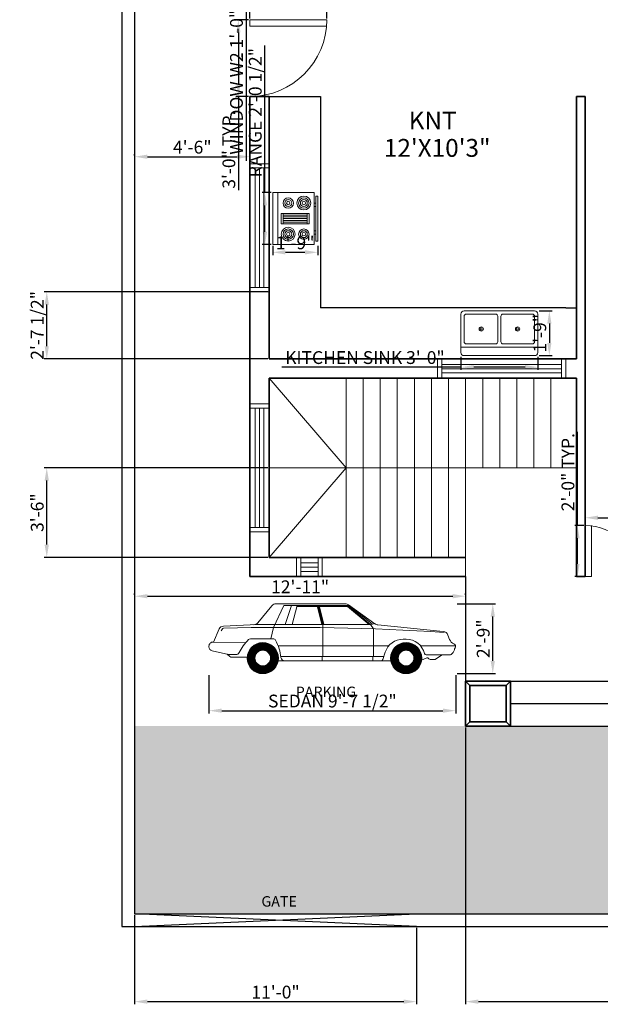
# Model space of a CAD drawing. Units: inches. Extents: x 104 to 647, y -91 to 674.
# Tile 1 of 3: x 104 to 376, y -91 to 371. Entities that reach past the tile are written whole.
import ezdxf

# ---------------------------------------------------------------- set-up
doc = ezdxf.new("R2010")
doc.units = ezdxf.units.IN
for name, color, linetype, lineweight in [('A-ANNO-DIMS', 2, 'Continuous', 18), ('A-ANNO-TEXT', 7, 'Continuous', 18), ('A-AREA-IDEN', 7, 'Continuous', 18), ('A-COLS', 7, 'Continuous', 35), ('A-DOOR', 3, 'Continuous', 18), ('A-EQPM', 8, 'Continuous', 18), ('A-FLOR', 7, 'Continuous', 25), ('A-FLOR-CASE', 8, 'Continuous', 25), ('A-FLOR-FIXT', 9, 'Continuous', 18), ('A-FLOR-STRS', 7, 'Continuous', 18), ('A-GLAZ', 4, 'Continuous', 18), ('A-WALL', 7, 'Continuous', 35), ('C-PKNG', 8, 'Continuous', 18), ('C-PROP', 7, 'Continuous', 25), ('L-PLNT-PATT', 3, 'Continuous', 13)]:
    doc.layers.add(name, color=color, linetype=linetype, lineweight=lineweight)
doc.styles.get("Standard").update_dxf_attribs({"font": 'arial.ttf'})
doc.dimstyles.new('ISO-25', dxfattribs={"dimtxt": 6, "dimasz": 6, "dimexe": 1.25, "dimexo": 0.625, "dimtad": 1, "dimdec": 1, "dimlunit": 3, "dimtxsty": 'Standard', "dimcen": 2.5, "dimadec": 0, "dimazin": 0, "dimtfac": 1, "dimtdec": 1, "dimtmove": 0, "dimatfit": 3, "dimfxl": 1, "dimarcsym": 0})

# ---------------------------------------------------------------- blocks, each defined once
blk = doc.blocks.new('Range-Oven - 30 in top')
for p, q in [((0, -3), (30, -3)), ((12, -6), (18, -6)), ((13, -20), (13, -6)), ((14, -6), (14, -20)), ((15, -20), (15, -6)), ((16, -6), (16, -20)), ((17, -20), (17, -6)), ((18, -20), (12, -20)), ((6, -24), (6, -25)), ((8, -25), (8, -24)), ((22, -25), (22, -24)), ((24, -24), (24, -25))]:
    blk.add_line(p, q)
for points in [[(0, -24), (0, 0), (30, 0), (30, -24)], [(12, -21), (12, -5), (18, -5), (18, -21)], [(2, -26), (2, -25), (28, -25), (28, -26)]]:
    blk.add_lwpolyline(points, close=True)
for centre, radius in [((6, -9), 4), ((6, -9), 3), ((6, -9), 2), ((6, -9), 1), ((24, -9), 3), ((24, -9), 2), ((24, -9), 1), ((6, -18), 3), ((6, -18), 2), ((6, -18), 1), ((24, -18), 4), ((24, -18), 3), ((24, -18), 2), ((24, -18), 1)]:
    blk.add_circle(centre, radius)
blk = doc.blocks.new('Sink-double - 36 in top')
for p, q in [((-18, -4), (18, -4)), ((-0.75, -18.5), (-0.75, -6.5)), ((0.75, -6.5), (0.75, -18.5))]:
    blk.add_line(p, q)
for points in [[(-16.5, 0), (16.5, 0)], [(-18, -19.5), (-18, -1.5)], [(18, -1.5), (18, -19.5)], [(-16.5, -18.5), (-16.5, -6.5)], [(-15.5, -5.5), (-1.75, -5.5)], [(1.75, -5.5), (15.5, -5.5)], [(16.5, -6.5), (16.5, -18.5)], [(16.5, -21), (-16.5, -21)], [(-1.75, -19.5), (-15.5, -19.5)], [(15.5, -19.5), (1.75, -19.5)]]:
    blk.add_lwpolyline(points)
for centre, radius in [((-8.5, -12.5), 1), ((-8.5, -12.5), 0.5), ((8.5, -12.5), 1), ((8.5, -12.5), 0.5)]:
    blk.add_circle(centre, radius)
for centre, radius, start, end in [((-16.5, -1.5), 1.5, 90, 180), ((16.5, -1.5), 1.5, 0, 90), ((-15.5, -6.5), 1, 90, 180), ((-1.75, -6.5), 1, 0, 90), ((1.75, -6.5), 1, 90, 180), ((15.5, -6.5), 1, 0, 90), ((-16.5, -19.5), 1.5, 180, 270), ((-15.5, -18.5), 1, 180, 270), ((-1.75, -18.5), 1, 270, 0), ((1.75, -18.5), 1, 180, 270), ((15.5, -18.5), 1, 270, 0), ((16.5, -19.5), 1.5, 270, 0)]:
    blk.add_arc(centre, radius, start, end)
blk = doc.blocks.new('Car - sedan  side')
for p, q in [((-77.81, 49.34), (-126.58, 49.34)), ((-139.53, 35.99), (-129.64, 47.91)), ((-128.57, 32.64), (-121.22, 48.02)), ((-74.7, 48.02), (-121.22, 48.02)), ((-120.32, 34.67), (-115.67, 48.02)), ((-115.4, 34.67), (-111.74, 48.02)), ((-97.55, 47.3), (-111.94, 47.3)), ((-94.41, 34.67), (-97.73, 48.02)), ((-93.72, 34.67), (-97.04, 48.02)), ((-93.03, 34.67), (-96.34, 48.02)), ((-76.26, 47.3), (-96.16, 47.3)), ((-61.08, 34.66), (-76.26, 47.3)), ((-60.02, 34.65), (-76.07, 48.02)), ((-56.87, 35.13), (-75.48, 48.59)), ((-58.54, 34.93), (-74.99, 48.02)), ((-60.02, 34.65), (-58.54, 34.93)), ((-57.21, 35.38), (-58.54, 34.93)), ((-170.93, 22.32), (-166.81, 31.56)), ((-164.57, 31.6), (-165.48, 30.35)), ((-140.23, 34.67), (-163.88, 33.56)), ((-62.28, 34.67), (-140.23, 34.67)), ((-130.39, 24.63), (-128.57, 32.64)), ((-93.72, 19.62), (-93.72, 34.67)), ((-62.28, 34.67), (-60.02, 34.65)), ((-57.97, 31.61), (-60.02, 34.65)), ((-57.97, 19.62), (-57.97, 31.61)), ((-54.93, 34.4), (-8.75, 29.8)), ((-148.26, 21.7), (-171.11, 22.33)), ((-128.78, 24.63), (-144.79, 24.63)), ((-36.97, 24.38), (-34.94, 24.38)), ((-4.21, 24.18), (-5.42, 27.27)), ((-174, 19.51), (-174, 18.91)), ((-160.12, 13.48), (-171.81, 16.16)), ((-47.2, 19.62), (-125.23, 19.62)), ((-93.72, 12.14), (-93.72, 19.62)), ((-57.97, 12.14), (-57.97, 19.62)), ((-51.4, 9.89), (-49.69, 15.14)), ((0, 19.62), (-24.7, 19.62)), ((-3.22, 13.59), (-1.77, 14.97)), ((-159.22, 12.14), (-161.08, 13.7)), ((-155.01, 13.48), (-160.12, 13.48)), ((-147.03, 11.6), (-157.73, 11.6)), ((-120.62, 9.03), (-125.23, 9.03)), ((-50.67, 12.14), (-123.32, 12.14)), ((-45.76, 9.03), (-120.62, 9.03)), ((-94.21, 9.03), (-94.21, 12.14)), ((-58.39, 9.03), (-58.39, 12.14)), ((-20.36, 11.06), (-24.06, 9.44)), ((-4.23, 13.19), (-20.72, 13.19)), ((-18.83, 10.42), (-19.11, 10.76)), ((-14.68, 10.03), (-18.01, 10.03)), ((-9.5, 13.19), (-14.1, 10.2))]:
    blk.add_line(p, q)
at = {"const_width": 5.49}
for points in [[(-127.8, 11, -1), (-144.3, 11, -1)], [(-26.69, 11, -1), (-43.19, 11, -1)]]:
    blk.add_lwpolyline(points, format="xyb", close=True, dxfattribs=at)
for centre, radius in [((-136.05, 11), 11), ((-34.94, 11), 11), ((-136.05, 11), 5.51), ((-34.94, 11), 5.51)]:
    blk.add_circle(centre, radius)
for centre, radius, start, end in [((-126.58, 45.38), 3.97, 90, 140.30288), ((-77.81, 45.38), 3.97, 54.13504, 90), ((-142.58, 38.53), 3.97, 272.68265, 320.30288), ((-54.54, 38.35), 3.97, 234.13503, 264.31231), ((-163.72, 30.18), 3.38, 92.68266, 155.97362), ((-163.62, 30.91), 1.17, 91.49105, 143.95527), ((-118.51, -1702.12), 1734.79, 86.34698, 91.49105), ((-9.15, 25.82), 4, 21.31069, 84.3123), ((-171.18, 19.51), 2.82, 88.41927, 180), ((-118.09, -2.78), 38.85, 136.3964, 152.90974), ((-144.79, 22.64), 1.98, 90, 136.3964), ((-128.78, 22.64), 1.98, 28.1371, 90), ((-157.14, 7.48), 34.14, 6.51354, 28.1371), ((-36.97, 11), 13.38, 90, 161.97316), ((-34.94, 11), 13.38, 13.58642, 90), ((0.9, 26.18), 5.49, 201.3107, 247.70484), ((-1.92, 19.3), 1.94, 325.37436, 67.70485), ((-171.18, 18.91), 2.82, 180, 257.09053), ((-155.01, 16.1), 2.62, 270, 332.90974), ((-20.72, 14.43), 1.24, 193.58641, 270), ((-3.82, 17.12), 2.96, 313.71735, 352.38387), ((2.46, 16.28), 3.37, 145.37437, 172.38386), ((-157.73, 13.93), 2.32, 230.12913, 270), ((-120.62, 11.65), 2.62, 186.51353, 270), ((-52.58, 10.27), 1.24, 270, 341.97316), ((-19.93, 10.09), 1.06, 39.30103, 113.71592), ((-18.01, 11.09), 1.06, 219.30104, 270), ((-14.68, 11.09), 1.06, 270, 303.04697), ((-4.23, 14.65), 1.46, 270, 313.71735)]:
    blk.add_arc(centre, radius, start, end)
blk = doc.blocks.new('*D9')
at = {"layer": 'A-ANNO-DIMS', "color": 0, "lineweight": -2, "transparency": 16777216}
for p, q in [((157.79, 307.2), (157.79, 307.83)), ((163.79, 306.58), (205.79, 306.58)), ((211.79, 191.42), (211.79, 307.83))]:
    blk.add_line(p, q, dxfattribs=at)
at = {"layer": 'A-ANNO-DIMS', "color": 0, "transparency": 16777216}
for points in [[(163.79, 307.58), (163.79, 305.58), (157.79, 306.58)], [(205.79, 307.58), (205.79, 305.58), (211.79, 306.58)]]:
    blk.add_solid(points, dxfattribs=at)
at = {"layer": 'Defpoints', "color": 0, "transparency": 16777216}
for p in [(157.79, 306.58), (211.79, 306.58), (211.79, 190.8)]:
    blk.add_point(p, dxfattribs=at)
at = {"layer": 'A-ANNO-DIMS', "color": 0, "transparency": 16777216, "insert": (184.79, 310.27), "char_height": 6, "attachment_point": 5}
blk.add_mtext('4\'-6"', dxfattribs=at)
blk = doc.blocks.new('*D13')
at = {"layer": 'A-ANNO-DIMS', "color": 0, "lineweight": -2, "transparency": 16777216}
for p, q in [((157.79, 101.27), (157.79, 101.89)), ((312.79, 101.27), (312.79, 101.89)), ((163.79, 100.64), (306.79, 100.64))]:
    blk.add_line(p, q, dxfattribs=at)
at = {"layer": 'A-ANNO-DIMS', "color": 0, "transparency": 16777216}
for points in [[(163.79, 101.64), (163.79, 99.64), (157.79, 100.64)], [(306.79, 101.64), (306.79, 99.64), (312.79, 100.64)]]:
    blk.add_solid(points, dxfattribs=at)
at = {"layer": 'Defpoints', "color": 0, "transparency": 16777216}
for p in [(157.79, 100.64), (312.79, 100.64), (312.79, 100.64)]:
    blk.add_point(p, dxfattribs=at)
at = {"layer": 'A-ANNO-DIMS', "color": 0, "transparency": 16777216, "insert": (235.29, 104.28), "char_height": 6, "attachment_point": 5}
blk.add_mtext('12\'-11"', dxfattribs=at)
blk = doc.blocks.new('WIN-60IN')
for p, q in [((60, 9), (0, 9)), ((0, 9), (0, 0)), ((2, 9), (2, 0)), ((2, 6.5), (58, 6.5)), ((58, 0), (58, 9)), ((60, 0), (60, 9)), ((0, 0), (60, 0)), ((2, 4.5), (58, 4.5)), ((2, 2.5), (58, 2.5))]:
    blk.add_line(p, q)
blk = doc.blocks.new('WIN-12IN')
for p, q in [((12, 9), (0, 9)), ((0, 9), (0, 0)), ((2, 9), (2, 0)), ((2, 6.5), (10, 6.5)), ((10, 0), (10, 9)), ((12, 0), (12, 9)), ((0, 0), (12, 0)), ((2, 4.5), (10, 4.5)), ((2, 2.5), (10, 2.5))]:
    blk.add_line(p, q)
blk = doc.blocks.new('DOOR-SWING-36IN')
for p, q in [((0, 3), (36, 3)), ((0, 0), (36, 0)), ((36, 0), (36, 3))]:
    blk.add_line(p, q)
blk.add_arc((36, 0), 36, 90, 180)
blk = doc.blocks.new('DOOR-ENTRY-LEAF-24IN')
for p, q in [((0, 24), (0, 0)), ((3, 24), (3, 0)), ((0, 0), (3, 0))]:
    blk.add_line(p, q)
blk.add_arc((0, 0), 24, 0, 90)
blk = doc.blocks.new('POST-21IN')
for p, q in [((0, 21), (2, 19)), ((19, 19), (21, 21)), ((0, 0), (2, 2)), ((19, 2), (21, 0))]:
    blk.add_line(p, q)
for points in [[(0, 0), (21, 0), (21, 21), (0, 21)], [(2, 2), (19, 2), (19, 19), (2, 19)]]:
    blk.add_lwpolyline(points, close=True)
blk = doc.blocks.new('*D29')
at = {"layer": 'A-ANNO-DIMS', "color": 0, "lineweight": -2, "transparency": 16777216}
for p, q in [((209.99, 426.8), (209.99, 432.8)), ((211.16, 420.8), (208.74, 420.8)), ((209.99, 420.8), (209.99, 408.8)), ((211.16, 408.8), (208.74, 408.8)), ((209.99, 402.8), (209.99, 304.72))]:
    blk.add_line(p, q, dxfattribs=at)
at = {"layer": 'A-ANNO-DIMS', "color": 0, "transparency": 16777216}
for points in [[(208.99, 426.8), (210.99, 426.8), (209.99, 420.8)], [(208.99, 402.8), (210.99, 402.8), (209.99, 408.8)]]:
    blk.add_solid(points, dxfattribs=at)
at = {"layer": 'Defpoints', "color": 0, "transparency": 16777216}
for p in [(211.79, 420.8), (209.99, 408.8), (211.79, 408.8)]:
    blk.add_point(p, dxfattribs=at)
at = {"layer": 'A-ANNO-DIMS', "color": 0, "transparency": 16777216, "insert": (206.26, 350.76), "char_height": 6, "attachment_point": 5, "rotation": 90}
blk.add_mtext('WINDOW W2 1\'-0" TYP.', dxfattribs=at)
blk = doc.blocks.new('*D31')
at = {"layer": 'A-ANNO-DIMS', "color": 0, "lineweight": -2, "transparency": 16777216}
for p, q in [((211.79, 376.2), (127.75, 376.2)), ((211.79, 371.42), (211.79, 377.45)), ((241.79, 376.2), (217.79, 376.2)), ((247.79, 371.42), (247.79, 377.45))]:
    blk.add_line(p, q, dxfattribs=at)
at = {"layer": 'A-ANNO-DIMS', "color": 0, "transparency": 16777216}
for points in [[(217.79, 377.2), (217.79, 375.2), (211.79, 376.2)], [(241.79, 377.2), (241.79, 375.2), (247.79, 376.2)]]:
    blk.add_solid(points, dxfattribs=at)
at = {"layer": 'Defpoints', "color": 0, "transparency": 16777216}
for p in [(211.79, 376.2), (211.79, 370.8), (247.79, 370.8)]:
    blk.add_point(p, dxfattribs=at)
at = {"layer": 'A-ANNO-DIMS', "color": 0, "transparency": 16777216, "insert": (166.77, 379.93), "char_height": 6, "attachment_point": 5}
blk.add_mtext('DOOR D1 3\'-0" TYP.', dxfattribs=at)
blk = doc.blocks.new('*D32')
at = {"layer": 'A-ANNO-DIMS', "color": 0, "lineweight": -2, "transparency": 16777216}
for p, q in [((211.16, 370.8), (205.14, 370.8)), ((206.39, 364.8), (206.39, 340.8)), ((211.16, 334.8), (205.14, 334.8)), ((206.39, 334.8), (206.39, 290.98))]:
    blk.add_line(p, q, dxfattribs=at)
at = {"layer": 'A-ANNO-DIMS', "color": 0, "transparency": 16777216}
for points in [[(205.39, 364.8), (207.39, 364.8), (206.39, 370.8)], [(205.39, 340.8), (207.39, 340.8), (206.39, 334.8)]]:
    blk.add_solid(points, dxfattribs=at)
at = {"layer": 'Defpoints', "color": 0, "transparency": 16777216}
for p in [(211.79, 370.8), (206.39, 334.8), (211.79, 334.8)]:
    blk.add_point(p, dxfattribs=at)
at = {"layer": 'A-ANNO-DIMS', "color": 0, "transparency": 16777216, "insert": (202.7, 309.89), "char_height": 6, "attachment_point": 5, "rotation": 90}
blk.add_mtext('3\'-0" TYP.', dxfattribs=at)
blk = doc.blocks.new('*D35')
at = {"layer": 'A-ANNO-DIMS', "color": 0, "lineweight": -2, "transparency": 16777216}
for p, q in [((368.79, 134.42), (368.79, 138.65)), ((392.79, 134.42), (392.79, 138.65)), ((374.79, 137.4), (386.79, 137.4)), ((392.79, 137.4), (490.32, 137.4))]:
    blk.add_line(p, q, dxfattribs=at)
at = {"layer": 'A-ANNO-DIMS', "color": 0, "transparency": 16777216}
for points in [[(374.79, 138.4), (374.79, 136.4), (368.79, 137.4)], [(386.79, 138.4), (386.79, 136.4), (392.79, 137.4)]]:
    blk.add_solid(points, dxfattribs=at)
at = {"layer": 'Defpoints', "color": 0, "transparency": 16777216}
for p in [(392.79, 137.4), (368.79, 133.8), (392.79, 133.8)]:
    blk.add_point(p, dxfattribs=at)
at = {"layer": 'A-ANNO-DIMS', "color": 0, "transparency": 16777216, "insert": (444.56, 141.09), "char_height": 6, "attachment_point": 5}
blk.add_mtext('ENTRY LEAF 2\'-0" TYP.', dxfattribs=at)
blk = doc.blocks.new('*D36')
at = {"layer": 'A-ANNO-DIMS', "color": 0, "lineweight": -2, "transparency": 16777216}
for p, q in [((365.19, 133.8), (365.19, 177.72)), ((368.16, 133.8), (363.94, 133.8)), ((365.19, 115.8), (365.19, 127.8)), ((368.16, 109.8), (363.94, 109.8))]:
    blk.add_line(p, q, dxfattribs=at)
at = {"layer": 'A-ANNO-DIMS', "color": 0, "transparency": 16777216}
for points in [[(364.19, 127.8), (366.19, 127.8), (365.19, 133.8)], [(364.19, 115.8), (366.19, 115.8), (365.19, 109.8)]]:
    blk.add_solid(points, dxfattribs=at)
at = {"layer": 'Defpoints', "color": 0, "transparency": 16777216}
for p in [(365.19, 133.8), (368.79, 133.8), (368.79, 109.8)]:
    blk.add_point(p, dxfattribs=at)
at = {"layer": 'A-ANNO-DIMS', "color": 0, "transparency": 16777216, "insert": (361.5, 158.76), "char_height": 6, "attachment_point": 5, "rotation": 90}
blk.add_mtext('2\'-0" TYP.', dxfattribs=at)
blk = doc.blocks.new('*D43')
at = {"layer": 'A-ANNO-DIMS', "color": 0, "lineweight": -2, "transparency": 16777216}
for p, q in [((218.79, 289.75), (218.79, 358.76)), ((221.81, 289.75), (217.54, 289.75)), ((218.79, 271.42), (218.79, 283.75)), ((221.81, 265.42), (217.54, 265.42))]:
    blk.add_line(p, q, dxfattribs=at)
at = {"layer": 'A-ANNO-DIMS', "color": 0, "transparency": 16777216}
for points in [[(217.79, 283.75), (219.79, 283.75), (218.79, 289.75)], [(217.79, 271.42), (219.79, 271.42), (218.79, 265.42)]]:
    blk.add_solid(points, dxfattribs=at)
at = {"layer": 'Defpoints', "color": 0, "transparency": 16777216}
for p in [(218.79, 289.75), (222.44, 289.75), (222.44, 265.42)]:
    blk.add_point(p, dxfattribs=at)
at = {"layer": 'A-ANNO-DIMS', "color": 0, "transparency": 16777216, "insert": (215.06, 327.25), "char_height": 6, "attachment_point": 5, "rotation": 90}
blk.add_mtext('RANGE 2\'-0 1/2"', dxfattribs=at)
blk = doc.blocks.new('*D44')
at = {"layer": 'A-ANNO-DIMS', "color": 0, "lineweight": -2, "transparency": 16777216}
for p, q in [((222.44, 264.79), (222.44, 260.52)), ((243.52, 264.79), (243.52, 260.52)), ((237.52, 261.77), (228.44, 261.77))]:
    blk.add_line(p, q, dxfattribs=at)
at = {"layer": 'A-ANNO-DIMS', "color": 0, "transparency": 16777216}
for points in [[(228.44, 262.77), (228.44, 260.77), (222.44, 261.77)], [(237.52, 262.77), (237.52, 260.77), (243.52, 261.77)]]:
    blk.add_solid(points, dxfattribs=at)
at = {"layer": 'Defpoints', "color": 0, "transparency": 16777216}
for p in [(222.44, 265.42), (243.52, 265.42), (222.44, 261.77)]:
    blk.add_point(p, dxfattribs=at)
at = {"layer": 'A-ANNO-DIMS', "color": 0, "transparency": 16777216, "insert": (232.98, 265.46), "char_height": 6, "attachment_point": 5}
blk.add_mtext('1\'-9"', dxfattribs=at)
blk = doc.blocks.new('*D45')
at = {"layer": 'A-ANNO-DIMS', "color": 0, "lineweight": -2, "transparency": 16777216}
for p, q in [((310.62, 212.74), (310.62, 206.71)), ((346.62, 212.74), (346.62, 206.71)), ((310.62, 207.96), (226.68, 207.96)), ((340.62, 207.96), (316.62, 207.96))]:
    blk.add_line(p, q, dxfattribs=at)
at = {"layer": 'A-ANNO-DIMS', "color": 0, "transparency": 16777216}
for points in [[(316.62, 208.96), (316.62, 206.96), (310.62, 207.96)], [(340.62, 208.96), (340.62, 206.96), (346.62, 207.96)]]:
    blk.add_solid(points, dxfattribs=at)
at = {"layer": 'Defpoints', "color": 0, "transparency": 16777216}
for p in [(310.62, 213.36), (346.62, 213.36), (310.62, 207.96)]:
    blk.add_point(p, dxfattribs=at)
at = {"layer": 'A-ANNO-DIMS', "color": 0, "transparency": 16777216, "insert": (265.65, 211.69), "char_height": 6, "attachment_point": 5}
blk.add_mtext('KITCHEN SINK 3\'-0"', dxfattribs=at)
blk = doc.blocks.new('*D46')
at = {"layer": 'A-ANNO-DIMS', "color": 0, "lineweight": -2, "transparency": 16777216}
for p, q in [((347.25, 234.36), (353.27, 234.36)), ((352.02, 228.36), (352.02, 219.36)), ((347.25, 213.36), (353.27, 213.36))]:
    blk.add_line(p, q, dxfattribs=at)
at = {"layer": 'A-ANNO-DIMS', "color": 0, "transparency": 16777216}
for points in [[(351.02, 228.36), (353.02, 228.36), (352.02, 234.36)], [(351.02, 219.36), (353.02, 219.36), (352.02, 213.36)]]:
    blk.add_solid(points, dxfattribs=at)
at = {"layer": 'Defpoints', "color": 0, "transparency": 16777216}
for p in [(346.62, 234.36), (346.62, 213.36), (352.02, 213.36)]:
    blk.add_point(p, dxfattribs=at)
at = {"layer": 'A-ANNO-DIMS', "color": 0, "transparency": 16777216, "insert": (348.33, 223.86), "char_height": 6, "attachment_point": 5, "rotation": 90}
blk.add_mtext('1\'-9"', dxfattribs=at)
blk = doc.blocks.new('*D49')
at = {"layer": 'A-ANNO-DIMS', "color": 0, "lineweight": -2, "transparency": 16777216}
for p, q in [((192.61, 63.71), (192.61, 45.75)), ((308.18, 63.71), (308.18, 45.75)), ((198.61, 47), (302.18, 47))]:
    blk.add_line(p, q, dxfattribs=at)
at = {"layer": 'A-ANNO-DIMS', "color": 0, "transparency": 16777216}
for points in [[(198.61, 48), (198.61, 46), (192.61, 47)], [(302.18, 48), (302.18, 46), (308.18, 47)]]:
    blk.add_solid(points, dxfattribs=at)
at = {"layer": 'Defpoints', "color": 0, "transparency": 16777216}
for p in [(192.61, 64.34), (308.18, 64.34), (308.18, 47)]:
    blk.add_point(p, dxfattribs=at)
at = {"layer": 'A-ANNO-DIMS', "color": 0, "transparency": 16777216, "insert": (250.4, 50.73), "char_height": 6, "attachment_point": 5}
blk.add_mtext('SEDAN 9\'-7 1/2"', dxfattribs=at)
blk = doc.blocks.new('*D50')
at = {"layer": 'A-ANNO-DIMS', "color": 0, "lineweight": -2, "transparency": 16777216}
for p, q in [((308.81, 97.09), (326.77, 97.09)), ((325.52, 70.34), (325.52, 91.09)), ((308.81, 64.34), (326.77, 64.34))]:
    blk.add_line(p, q, dxfattribs=at)
at = {"layer": 'A-ANNO-DIMS', "color": 0, "transparency": 16777216}
for points in [[(324.52, 91.09), (326.52, 91.09), (325.52, 97.09)], [(324.52, 70.34), (326.52, 70.34), (325.52, 64.34)]]:
    blk.add_solid(points, dxfattribs=at)
at = {"layer": 'Defpoints', "color": 0, "transparency": 16777216}
for p in [(308.18, 97.09), (325.52, 97.09), (308.18, 64.34)]:
    blk.add_point(p, dxfattribs=at)
at = {"layer": 'A-ANNO-DIMS', "color": 0, "transparency": 16777216, "insert": (321.83, 80.71), "char_height": 6, "attachment_point": 5, "rotation": 90}
blk.add_mtext('2\'-9"', dxfattribs=at)
blk = doc.blocks.new('*D53')
at = {"layer": 'A-ANNO-DIMS', "color": 0, "lineweight": -2, "transparency": 16777216}
for p, q in [((312.79, 39.17), (312.79, -90.6)), ((545.79, 39.17), (545.79, -90.6)), ((318.79, -89.35), (539.79, -89.35))]:
    blk.add_line(p, q, dxfattribs=at)
at = {"layer": 'A-ANNO-DIMS', "color": 0, "transparency": 16777216}
for points in [[(318.79, -88.35), (318.79, -90.35), (312.79, -89.35)], [(539.79, -88.35), (539.79, -90.35), (545.79, -89.35)]]:
    blk.add_solid(points, dxfattribs=at)
at = {"layer": 'Defpoints', "color": 0, "transparency": 16777216}
for p in [(312.79, 39.8), (545.79, 39.8), (545.79, -89.35)]:
    blk.add_point(p, dxfattribs=at)
at = {"layer": 'A-ANNO-DIMS', "color": 0, "transparency": 16777216, "insert": (429.29, -85.66), "char_height": 6, "attachment_point": 5}
blk.add_mtext('19\'-5"', dxfattribs=at)
blk = doc.blocks.new('*D55')
at = {"layer": 'A-ANNO-DIMS', "color": 0, "lineweight": -2, "transparency": 16777216}
for p, q in [((157.79, -48.83), (157.79, -90.6)), ((289.79, -54.83), (289.79, -90.6)), ((163.79, -89.35), (283.79, -89.35))]:
    blk.add_line(p, q, dxfattribs=at)
at = {"layer": 'A-ANNO-DIMS', "color": 0, "transparency": 16777216}
for points in [[(163.79, -88.35), (163.79, -90.35), (157.79, -89.35)], [(283.79, -88.35), (283.79, -90.35), (289.79, -89.35)]]:
    blk.add_solid(points, dxfattribs=at)
at = {"layer": 'Defpoints', "color": 0, "transparency": 16777216}
for p in [(157.79, -48.2), (289.79, -54.2), (289.79, -89.35)]:
    blk.add_point(p, dxfattribs=at)
at = {"layer": 'A-ANNO-DIMS', "color": 0, "transparency": 16777216, "insert": (223.79, -85.66), "char_height": 6, "attachment_point": 5}
blk.add_mtext('11\'-0"', dxfattribs=at)
blk = doc.blocks.new('*D56')
at = {"layer": 'A-ANNO-DIMS', "color": 0, "lineweight": -2, "transparency": 16777216}
for p, q in [((220.16, 160.8), (115.39, 160.8)), ((116.64, 124.8), (116.64, 154.8)), ((220.16, 118.8), (115.39, 118.8))]:
    blk.add_line(p, q, dxfattribs=at)
at = {"layer": 'A-ANNO-DIMS', "color": 0, "transparency": 16777216}
for points in [[(115.64, 154.8), (117.64, 154.8), (116.64, 160.8)], [(115.64, 124.8), (117.64, 124.8), (116.64, 118.8)]]:
    blk.add_solid(points, dxfattribs=at)
at = {"layer": 'Defpoints', "color": 0, "transparency": 16777216}
for p in [(116.64, 160.8), (220.79, 160.8), (220.79, 118.8)]:
    blk.add_point(p, dxfattribs=at)
at = {"layer": 'A-ANNO-DIMS', "color": 0, "transparency": 16777216, "insert": (112.95, 139.8), "char_height": 6, "attachment_point": 5, "rotation": 90}
blk.add_mtext('3\'-6"', dxfattribs=at)
blk = doc.blocks.new('*D58')
at = {"layer": 'A-ANNO-DIMS', "color": 0, "lineweight": -2, "transparency": 16777216}
for p, q in [((220.16, 243.3), (115.39, 243.3)), ((116.64, 217.8), (116.64, 237.3)), ((220.16, 211.8), (115.39, 211.8))]:
    blk.add_line(p, q, dxfattribs=at)
at = {"layer": 'A-ANNO-DIMS', "color": 0, "transparency": 16777216}
for points in [[(115.64, 237.3), (117.64, 237.3), (116.64, 243.3)], [(115.64, 217.8), (117.64, 217.8), (116.64, 211.8)]]:
    blk.add_solid(points, dxfattribs=at)
at = {"layer": 'Defpoints', "color": 0, "transparency": 16777216}
for p in [(116.64, 243.3), (220.79, 243.3), (220.79, 211.8)]:
    blk.add_point(p, dxfattribs=at)
at = {"layer": 'A-ANNO-DIMS', "color": 0, "transparency": 16777216, "insert": (112.91, 227.55), "char_height": 6, "attachment_point": 5, "rotation": 90}
blk.add_mtext('2\'-7 1/2"', dxfattribs=at)

msp = doc.modelspace()

# ---------------------------------------------------------------- hatches: boundary and pattern name
at = {"layer": 'L-PLNT-PATT'}
h = msp.add_hatch(dxfattribs=at)
h.set_pattern_fill('GRASS', color=256, scale=0.2)
h.paths.add_polyline_path([(569.79, 39.8), (546.01, 39.8), (524.79, 39.8), (312.79, 39.8), (157.79, 39.8), (157.79, -48.2), (205.79, -48.2), (545.79, -48.2), (569.79, -48.2)])

# ---------------------------------------------------------------- linework, layer by layer
at = {"layer": 'A-FLOR'}
for p, q in [((312.79, 109.8), (312.79, 39.8)), ((312.79, 60.8), (545.79, 60.8)), ((333.79, 50.3), (524.79, 50.3)), ((312.79, 39.8), (545.79, 39.8))]:
    msp.add_line(p, q, dxfattribs=at)
at = {"layer": 'A-FLOR-CASE'}
for p, q in [((220.79, 334.8), (244.79, 334.8)), ((244.79, 334.8), (244.79, 235.8)), ((308.79, 235.8), (244.79, 235.8)), ((359.67, 235.74), (299.67, 235.74)), ((359.67, 235.74), (364.79, 235.74))]:
    msp.add_line(p, q, dxfattribs=at)
at = {"layer": 'A-FLOR-STRS'}
for p, q in [((256.79, 160.8), (220.79, 202.8)), ((256.79, 202.8), (256.79, 118.8)), ((264.79, 202.8), (264.79, 118.8)), ((272.79, 202.8), (272.79, 118.8)), ((280.79, 202.8), (280.79, 118.8)), ((288.79, 202.8), (288.79, 118.8)), ((296.79, 202.8), (296.79, 118.8)), ((304.79, 202.8), (304.79, 118.8)), ((312.79, 202.8), (312.79, 109.8)), ((320.79, 202.8), (320.79, 160.8)), ((328.79, 202.8), (328.79, 160.8)), ((336.79, 202.8), (336.79, 160.8)), ((344.79, 202.8), (344.79, 160.8)), ((352.79, 202.8), (352.79, 160.8)), ((256.79, 160.8), (220.79, 160.8)), ((220.79, 118.8), (256.79, 160.8)), ((256.79, 160.8), (364.79, 160.8))]:
    msp.add_line(p, q, dxfattribs=at)
at = {"layer": 'A-WALL'}
for p, q in [((220.79, 334.8), (211.79, 334.8)), ((211.79, 334.8), (211.79, 109.8)), ((220.79, 334.8), (220.79, 211.8)), ((368.79, 334.8), (364.79, 334.8)), ((364.79, 334.8), (364.79, 211.8)), ((368.79, 334.8), (368.79, 109.8)), ((308.79, 211.8), (220.79, 211.8)), ((308.79, 211.8), (364.79, 211.8)), ((308.79, 202.8), (220.79, 202.8)), ((220.79, 202.8), (220.79, 118.8)), ((308.79, 202.8), (364.79, 202.8)), ((364.79, 202.8), (364.79, 109.8)), ((312.79, 118.8), (220.79, 118.8)), ((312.79, 109.8), (211.79, 109.8)), ((368.79, 109.8), (364.79, 109.8))]:
    msp.add_line(p, q, dxfattribs=at)
at = {"layer": 'C-PROP'}
for p, q in [((151.79, 617.8), (151.79, -54.2)), ((157.79, 608.8), (157.79, -48.2)), ((157.79, -48.2), (205.79, -48.2)), ((157.79, -54.2), (289.79, -48.2)), ((289.79, -54.2), (157.79, -48.2)), ((205.79, -48.2), (545.79, -48.2)), ((151.79, -54.2), (205.79, -54.2)), ((205.79, -54.2), (545.79, -54.2))]:
    msp.add_line(p, q, dxfattribs=at)

# ---------------------------------------------------------------- block references
at = {"layer": 'A-COLS'}
msp.add_blockref('POST-21IN', (312.79, 39.8), dxfattribs=at)
at = {"layer": 'A-DOOR', "rotation": 180}
msp.add_blockref('DOOR-SWING-36IN', (247.79, 370.8), dxfattribs=at)
at = {"layer": 'A-DOOR'}
msp.add_blockref('DOOR-ENTRY-LEAF-24IN', (368.79, 109.8), dxfattribs=at)
at = {"layer": 'A-EQPM', "xscale": 0.8110349602000754, "yscale": 0.8110349602000754, "zscale": 0.8110349602000754, "rotation": 90}
msp.add_blockref('Range-Oven - 30 in top', (222.44, 265.42), dxfattribs=at)
at = {"layer": 'A-FLOR-FIXT', "rotation": 180}
msp.add_blockref('Sink-double - 36 in top', (328.62, 213.36), dxfattribs=at)
at = {"layer": 'A-GLAZ'}
for p, rotation in [((220.79, 243.3), 90.00000000000003), ((359.67, 211.74), 180), ((220.79, 130.8), 90.00000000000006)]:
    msp.add_blockref('WIN-60IN', p, dxfattribs=dict(at, rotation=rotation))
msp.add_blockref('WIN-12IN', (233.67, 109.75), dxfattribs=at)
at = {"layer": 'C-PKNG', "xscale": 0.6637563944722635, "yscale": 0.6637563944722635, "zscale": 0.6637563944722635}
msp.add_blockref('Car - sedan  side', (308.11, 64.34), dxfattribs=at)

# ---------------------------------------------------------------- texts
at = {"layer": 'A-ANNO-TEXT', "insert": (217.16, -39.92), "char_height": 4.906, "attachment_point": 1}
msp.add_mtext_dynamic_manual_height_columns('GATE', width=132.3228, gutter_width=24.53, heights=[0], dxfattribs=at)
at = {"layer": 'A-AREA-IDEN', "attachment_point": 1}
for s, width, gutter_width, insert, char_height in [('KNT', 225.5639, 41.81, (286.15, 327.71), 8.362), ('12\'X10\'3"', 225.5639, 41.81, (274.53, 314.91), 8.362), ('PARKING', 132.3228, 24.53, (233.25, 58.25), 4.906)]:
    msp.add_mtext_dynamic_manual_height_columns(s, width=width, gutter_width=gutter_width, heights=[0], dxfattribs=dict(at, insert=insert, char_height=char_height))

# ---------------------------------------------------------------- dimensions: what is measured, and where the dimension line sits
at = {"layer": 'A-ANNO-DIMS'}
for base, p1, p2, angle, text, picture, middle in [((209.99, 408.8), (211.79, 420.8), (211.79, 408.8), 270, 'WINDOW W2 <> TYP.', '*D29', (206.26, 350.76)), ((211.79, 376.2), (247.79, 370.8), (211.79, 370.8), 180, 'DOOR D1 <> TYP.', '*D31', (166.77, 379.93)), ((206.39, 334.8), (211.79, 370.8), (211.79, 334.8), 270, '<> TYP.', '*D32', (202.7, 309.89)), ((218.79, 289.75), (222.44, 265.42), (222.44, 289.75), 90, 'RANGE <>', '*D43', (215.06, 327.25)), ((310.62, 207.96), (346.62, 213.36), (310.62, 213.36), 180, 'KITCHEN SINK <>', '*D45', (265.65, 211.69)), ((365.19, 133.8), (368.79, 109.8), (368.79, 133.8), 90, '<> TYP.', '*D36', (361.5, 158.76))]:
    dim = msp.add_linear_dim(base=base, p1=p1, p2=p2, angle=angle, text=text, dimstyle='ISO-25', override={"dimdec": 1, "dimlfac": 1, "dimrnd": 0, "dimzin": 1, "dimdsep": 46, "dimlunit": 4, "dimfrac": 2}, dxfattribs=at)
    dim.commit()
    dim.dimension.update_dxf_attribs({"geometry": picture, "text_midpoint": middle})
for base, p1, p2, override, picture, middle in [((211.79, 306.58), (157.79, 306.58), (211.79, 190.8), {"dimclrd": 0, "dimclre": 0, "dimclrt": 0}, '*D9', (184.79, 310.27)), ((312.79, 100.64), (157.79, 100.64), (312.79, 100.64), {"dimclrd": 0, "dimclre": 0, "dimclrt": 0}, '*D13', (235.29, 104.28)), ((545.79, -89.35), (312.79, 39.8), (545.79, 39.8), {"dimdec": 1, "dimlfac": 1, "dimrnd": 0, "dimzin": 1, "dimdsep": 46, "dimlunit": 4, "dimfrac": 2}, '*D53', (429.29, -85.66)), ((289.79, -89.35), (157.79, -48.2), (289.79, -54.2), {"dimdec": 1, "dimlfac": 1, "dimrnd": 0, "dimzin": 1, "dimdsep": 46, "dimlunit": 4, "dimfrac": 2}, '*D55', (223.79, -85.66))]:
    dim = msp.add_linear_dim(base=base, p1=p1, p2=p2, dimstyle='ISO-25', override=override, dxfattribs=at)
    dim.commit()
    dim.dimension.update_dxf_attribs({"geometry": picture, "text_midpoint": middle})
for base, p1, p2, angle, picture, middle in [((222.44, 261.77), (243.52, 265.42), (222.44, 265.42), 180, '*D44', (232.98, 265.46)), ((116.64, 243.3), (220.79, 211.8), (220.79, 243.3), 90, '*D58', (112.91, 227.55)), ((352.02, 213.36), (346.62, 234.36), (346.62, 213.36), 270, '*D46', (348.33, 223.86)), ((116.64, 160.8), (220.79, 118.8), (220.79, 160.8), 90, '*D56', (112.95, 139.8)), ((325.5192, 97.0894), (308.1839, 64.3364), (308.1839, 97.0894), 90, '*D50', (321.8308, 80.7129))]:
    dim = msp.add_linear_dim(base=base, p1=p1, p2=p2, angle=angle, dimstyle='ISO-25', override={"dimdec": 1, "dimlfac": 1, "dimrnd": 0, "dimzin": 1, "dimdsep": 46, "dimlunit": 4, "dimfrac": 2}, dxfattribs=at)
    dim.commit()
    dim.dimension.update_dxf_attribs({"geometry": picture, "text_midpoint": middle})
for base, p1, p2, text, picture, middle in [((392.79, 137.4), (368.79, 133.8), (392.79, 133.8), 'ENTRY LEAF <> TYP.', '*D35', (444.56, 141.09)), ((308.18, 47), (192.61, 64.34), (308.18, 64.34), 'SEDAN <>', '*D49', (250.4, 50.73))]:
    dim = msp.add_linear_dim(base=base, p1=p1, p2=p2, text=text, dimstyle='ISO-25', override={"dimdec": 1, "dimlfac": 1, "dimrnd": 0, "dimzin": 1, "dimdsep": 46, "dimlunit": 4, "dimfrac": 2}, dxfattribs=at)
    dim.commit()
    dim.dimension.update_dxf_attribs({"geometry": picture, "text_midpoint": middle})

doc.saveas('drawing.dxf')
